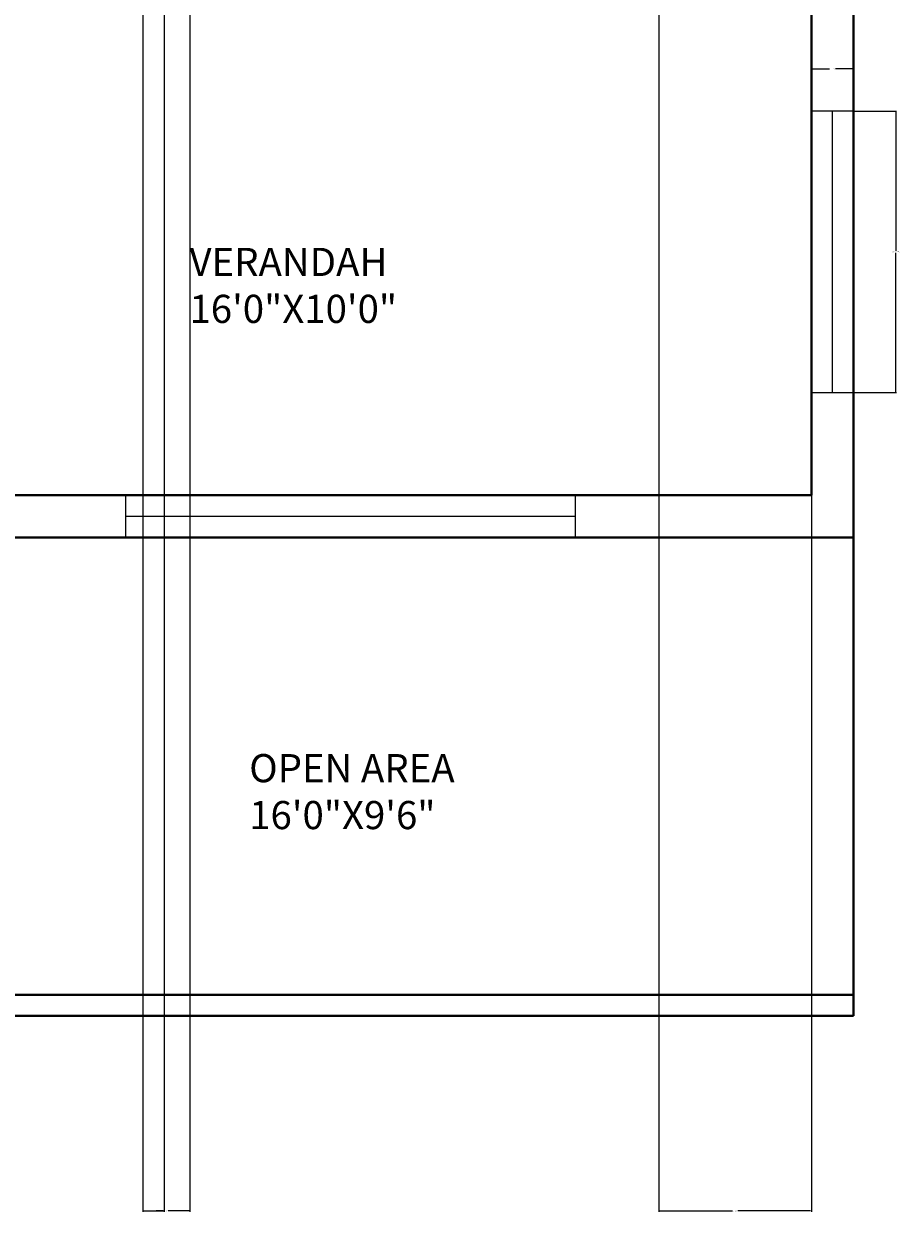
# Model space of a CAD drawing. Units: inches. Extents: x -19 to 419, y -828 to 43.
# Tile 5 of 9: x 233 to 419, y -828 to -574. Entities that reach past the tile are written whole.
import ezdxf

# ---------------------------------------------------------------- set-up
doc = ezdxf.new("R2010")
doc.units = ezdxf.units.IN
doc.header["$MEASUREMENT"] = 0
for name, color, linetype, lineweight in [('A-ANNO-DIMS', 2, 'Continuous', 18), ('A-AREA-IDEN', 7, 'Continuous', 25), ('A-GLAZ', 4, 'Continuous', 20), ('A-WALL', 7, 'Continuous', 40)]:
    doc.layers.add(name, color=color, linetype=linetype, lineweight=lineweight)
doc.styles.get("Standard").update_dxf_attribs({"font": 'arial.ttf'})
doc.dimstyles.get("Standard").update_dxf_attribs({"dimtxt": 0.18, "dimasz": 0.18, "dimexe": 0.18, "dimexo": 0.0625, "dimgap": 0.09, "dimtad": 0, "dimtih": 1, "dimtoh": 1, "dimdec": 0, "dimzin": 0, "dimdsep": 46, "dimlunit": 3, "dimtxsty": 'Standard', "dimcen": 0.09, "dimadec": 0, "dimazin": 0, "dimtfac": 1, "dimtdec": 0, "dimtofl": 0, "dimtmove": 0, "dimatfit": 3, "dimfxl": 1, "dimtolj": 1, "dimtzin": 0, "dimarcsym": 0})

# ---------------------------------------------------------------- blocks, each defined once
blk = doc.blocks.new('WIN-96X9')
for p, q in [((96, 9), (0, 9)), ((0, 9), (0, 0)), ((96, 0), (96, 9)), ((0, 4.5), (96, 4.5)), ((0, 0), (96, 0))]:
    blk.add_line(p, q)
blk = doc.blocks.new('WIN-60X9')
for p, q in [((60, 9), (0, 9)), ((0, 9), (0, 0)), ((60, 0), (60, 9)), ((0, 4.5), (60, 4.5)), ((0, 0), (60, 0))]:
    blk.add_line(p, q)
blk = doc.blocks.new('*D18')
at = {"layer": 'A-ANNO-DIMS', "color": 0, "lineweight": -2, "transparency": 16777216}
for p, q in [((409.8, -592.86), (418.92, -592.86)), ((418.74, -593.04), (418.74, -622.67)), ((418.74, -652.68), (418.74, -623.04)), ((409.8, -652.86), (418.92, -652.86))]:
    blk.add_line(p, q, dxfattribs=at)
at = {"layer": 'A-ANNO-DIMS', "color": 0, "transparency": 16777216}
for points in [[(418.71, -593.04), (418.77, -593.04), (418.74, -592.86)], [(418.71, -652.68), (418.77, -652.68), (418.74, -652.86)]]:
    blk.add_solid(points, dxfattribs=at)
at = {"layer": 'Defpoints', "color": 0, "transparency": 16777216}
for p in [(409.74, -592.86), (418.74, -592.86), (409.74, -652.86)]:
    blk.add_point(p, dxfattribs=at)
at = {"layer": 'A-ANNO-DIMS', "color": 0, "transparency": 16777216, "insert": (418.74, -622.86), "char_height": 0.18, "attachment_point": 5}
blk.add_mtext('\\A1;W2 5\'-0" TYP.', dxfattribs=at)
blk = doc.blocks.new('*D19')
at = {"layer": 'A-ANNO-DIMS', "color": 0, "lineweight": -2, "transparency": 16777216}
for p, q in [((400.74, -592.79), (400.74, -583.68)), ((400.92, -583.86), (404.6, -583.86)), ((409.56, -583.86), (405.88, -583.86)), ((409.74, -592.79), (409.74, -583.68))]:
    blk.add_line(p, q, dxfattribs=at)
at = {"layer": 'A-ANNO-DIMS', "color": 0, "transparency": 16777216}
for points in [[(400.92, -583.83), (400.92, -583.89), (400.74, -583.86)], [(409.56, -583.83), (409.56, -583.89), (409.74, -583.86)]]:
    blk.add_solid(points, dxfattribs=at)
at = {"layer": 'Defpoints', "color": 0, "transparency": 16777216}
for p in [(400.74, -583.86), (400.74, -592.86), (409.74, -592.86)]:
    blk.add_point(p, dxfattribs=at)
at = {"layer": 'A-ANNO-DIMS', "color": 0, "transparency": 16777216, "insert": (405.24, -583.86), "char_height": 0.18, "attachment_point": 5}
blk.add_mtext('\\A1;0\'-9" TYP.', dxfattribs=at)
blk = doc.blocks.new('*D45')
at = {"layer": 'A-ANNO-DIMS', "color": 0, "lineweight": -2, "transparency": 16777216}
for p, q in [((258.24, -550.3), (258.24, -827.51)), ((268.24, -550.3), (268.24, -827.51)), ((258.42, -827.33), (262.84, -827.33)), ((268.06, -827.33), (263.64, -827.33))]:
    blk.add_line(p, q, dxfattribs=at)
at = {"layer": 'A-ANNO-DIMS', "color": 0, "transparency": 16777216}
for points in [[(258.42, -827.3), (258.42, -827.36), (258.24, -827.33)], [(268.06, -827.3), (268.06, -827.36), (268.24, -827.33)]]:
    blk.add_solid(points, dxfattribs=at)
at = {"layer": 'Defpoints', "color": 0, "transparency": 16777216}
for p in [(258.24, -550.23), (268.24, -550.23), (268.24, -827.33)]:
    blk.add_point(p, dxfattribs=at)
at = {"layer": 'A-ANNO-DIMS', "color": 0, "transparency": 16777216, "insert": (263.24, -827.33), "char_height": 0.18, "attachment_point": 5}
blk.add_mtext('\\A1;0\'-10"', dxfattribs=at)
blk = doc.blocks.new('*D46')
at = {"layer": 'A-ANNO-DIMS', "color": 0, "lineweight": -2, "transparency": 16777216}
for p, q in [((368.24, -550.3), (368.24, -827.51)), ((400.74, -550.3), (400.74, -827.51)), ((368.42, -827.33), (383.95, -827.33)), ((400.56, -827.33), (385.03, -827.33))]:
    blk.add_line(p, q, dxfattribs=at)
at = {"layer": 'A-ANNO-DIMS', "color": 0, "transparency": 16777216}
for points in [[(368.42, -827.3), (368.42, -827.36), (368.24, -827.33)], [(400.56, -827.3), (400.56, -827.36), (400.74, -827.33)]]:
    blk.add_solid(points, dxfattribs=at)
at = {"layer": 'Defpoints', "color": 0, "transparency": 16777216}
for p in [(368.24, -550.23), (400.74, -550.23), (400.74, -827.33)]:
    blk.add_point(p, dxfattribs=at)
at = {"layer": 'A-ANNO-DIMS', "color": 0, "transparency": 16777216, "insert": (384.49, -827.33), "char_height": 0.18, "attachment_point": 5}
blk.add_mtext('\\A1;2\'-8 1/2"', dxfattribs=at)
blk = doc.blocks.new('*D48')
at = {"layer": 'A-ANNO-DIMS', "color": 0, "lineweight": -2, "transparency": 16777216}
for p, q in [((258.24, -473.8), (258.24, -827.51)), ((262.74, -473.8), (262.74, -827.51)), ((258.42, -827.33), (259.95, -827.33)), ((262.56, -827.33), (261.03, -827.33))]:
    blk.add_line(p, q, dxfattribs=at)
at = {"layer": 'A-ANNO-DIMS', "color": 0, "transparency": 16777216}
for points in [[(258.42, -827.3), (258.42, -827.36), (258.24, -827.33)], [(262.56, -827.3), (262.56, -827.36), (262.74, -827.33)]]:
    blk.add_solid(points, dxfattribs=at)
at = {"layer": 'Defpoints', "color": 0, "transparency": 16777216}
for p in [(258.24, -473.73), (262.74, -473.73), (262.74, -827.33)]:
    blk.add_point(p, dxfattribs=at)
at = {"layer": 'A-ANNO-DIMS', "color": 0, "transparency": 16777216, "insert": (260.49, -827.33), "char_height": 0.18, "attachment_point": 5}
blk.add_mtext('\\A1;0\'-4 1/2"', dxfattribs=at)

msp = doc.modelspace()

# ---------------------------------------------------------------- linework, layer by layer
at = {"layer": 'A-WALL'}
for p, q in [((409.74, -259.23), (409.74, -785.73)), ((400.74, -554.73), (400.74, -674.73)), ((204.24, -674.73), (400.74, -674.73)), ((195.24, -683.73), (400.74, -683.73)), ((400.74, -683.73), (409.74, -683.73)), ((22.74, -781.23), (409.74, -781.23)), ((22.74, -785.73), (409.74, -785.73))]:
    msp.add_line(p, q, dxfattribs=at)

# ---------------------------------------------------------------- block references
at = {"layer": 'A-GLAZ', "rotation": 90.00000000000021}
msp.add_blockref('WIN-60X9', (409.74, -652.86), dxfattribs=at)
at = {"layer": 'A-GLAZ'}
msp.add_blockref('WIN-96X9', (254.49, -683.73), dxfattribs=at)

# ---------------------------------------------------------------- texts
at = {"layer": 'A-AREA-IDEN', "char_height": 6, "attachment_point": 1}
for s, insert in [('VERANDAH\\P16\'0"X10\'0"', (268.16, -622.01)), ('OPEN AREA\\P16\'0"X9\'6"', (280.89, -729.93))]:
    msp.add_mtext(s, dxfattribs=dict(at, insert=insert))

# ---------------------------------------------------------------- dimensions: what is measured, and where the dimension line sits
at = {"layer": 'A-ANNO-DIMS'}
for base, p1, p2, picture, middle in [((262.74, -827.33), (258.24, -473.73), (262.74, -473.73), '*D48', (260.49, -827.33)), ((268.24, -827.33), (258.24, -550.23), (268.24, -550.23), '*D45', (263.24, -827.33)), ((400.74, -827.33), (368.24, -550.23), (400.74, -550.23), '*D46', (384.49, -827.33))]:
    dim = msp.add_linear_dim(base=base, p1=p1, p2=p2, dimstyle='Standard', override={"dimdec": 1, "dimlfac": 1, "dimrnd": 0, "dimzin": 1, "dimdsep": 46, "dimlunit": 4, "dimfrac": 2}, dxfattribs=at)
    dim.commit()
    dim.dimension.update_dxf_attribs({"geometry": picture, "text_midpoint": middle})
for base, p1, p2, angle, text, picture, middle in [((400.74, -583.86), (409.74, -592.86), (400.74, -592.86), 180, '<> TYP.', '*D19', (405.24, -583.86)), ((418.74, -592.86), (409.74, -652.86), (409.74, -592.86), 90, 'W2 <> TYP.', '*D18', (418.74, -622.86))]:
    dim = msp.add_linear_dim(base=base, p1=p1, p2=p2, angle=angle, text=text, dimstyle='Standard', override={"dimdec": 1, "dimlfac": 1, "dimrnd": 0, "dimzin": 1, "dimdsep": 46, "dimlunit": 4, "dimfrac": 2}, dxfattribs=at)
    dim.commit()
    dim.dimension.update_dxf_attribs({"geometry": picture, "text_midpoint": middle})

doc.saveas('drawing.dxf')
